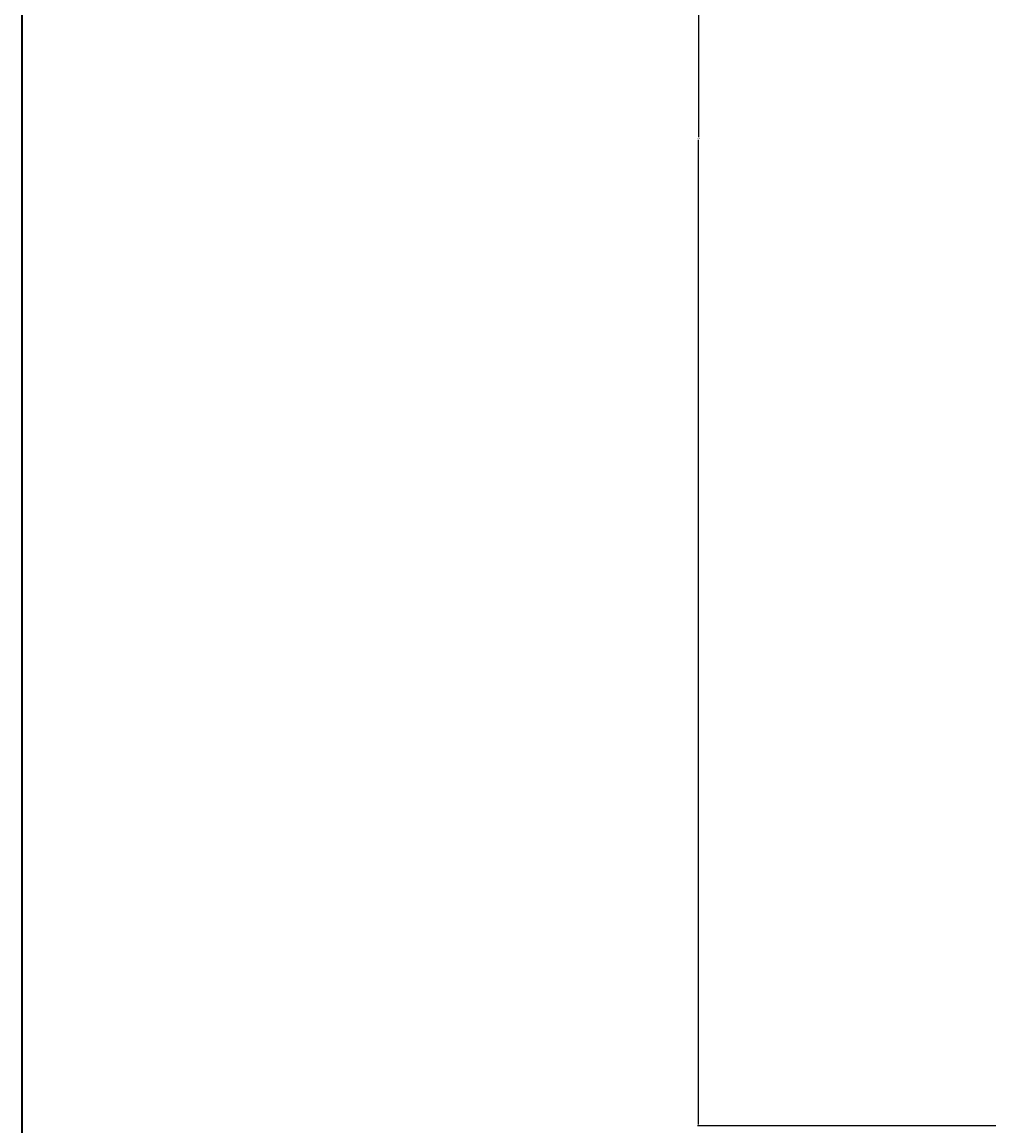
# Model space of a CAD drawing. Units: inches. Extents: x 2120 to 4013, y 1390 to 3019.
# Tile 1 of 59: x 2120 to 2259, y 1582 to 1740. Entities that reach past the tile are written whole.
import ezdxf

# ---------------------------------------------------------------- set-up
doc = ezdxf.new("R2010")
doc.units = ezdxf.units.IN
doc.layers.add('A-ANNO-DIMS', color=2, linetype='Continuous', lineweight=18)
doc.layers.add('A-ANNO-TTLB', color=7, linetype='Continuous', lineweight=35)
doc.styles.get("Standard").update_dxf_attribs({"font": 'arial.ttf'})
doc.dimstyles.get("Standard").update_dxf_attribs({"dimtxt": 0.18, "dimasz": 0.18, "dimexe": 0.18, "dimexo": 0.0625, "dimgap": 0.09, "dimtad": 0, "dimtih": 1, "dimtoh": 1, "dimdec": 4, "dimzin": 0, "dimdsep": 46, "dimtxsty": 'Standard', "dimcen": 0.09, "dimadec": 0, "dimazin": 0, "dimtfac": 1, "dimtdec": 4, "dimtofl": 0, "dimtmove": 0, "dimatfit": 3, "dimfxl": 1, "dimtolj": 1, "dimtzin": 0, "dimarcsym": 0})

# ---------------------------------------------------------------- blocks, each defined once
blk = doc.blocks.new('*D213')
at = {"layer": 'A-ANNO-DIMS', "color": 0, "lineweight": -2, "transparency": 16777216}
for p, q in [((2271.67, 1865.53), (2217.55, 1865.53)), ((2217.73, 1865.35), (2217.73, 1723.71)), ((2217.73, 1581.71), (2217.73, 1723.35)), ((2262.67, 1581.53), (2217.55, 1581.53))]:
    blk.add_line(p, q, dxfattribs=at)
at = {"layer": 'A-ANNO-DIMS', "color": 0, "transparency": 16777216}
for points in [[(2217.7, 1865.35), (2217.76, 1865.35), (2217.73, 1865.53)], [(2217.7, 1581.71), (2217.76, 1581.71), (2217.73, 1581.53)]]:
    blk.add_solid(points, dxfattribs=at)
at = {"layer": 'Defpoints', "color": 0, "transparency": 16777216}
for p in [(2217.73, 1865.53), (2271.73, 1865.53), (2262.73, 1581.53)]:
    blk.add_point(p, dxfattribs=at)
at = {"layer": 'A-ANNO-DIMS', "color": 0, "transparency": 16777216, "insert": (2217.73, 1723.53), "char_height": 0.18, "attachment_point": 5}
blk.add_mtext('\\A1;284', dxfattribs=at)

msp = doc.modelspace()

# ---------------------------------------------------------------- linework, layer by layer
at = {"layer": 'A-ANNO-TTLB'}
msp.add_lwpolyline([(2120.4581, 3019.1237), (4012.9334, 3019.1237), (4012.9334, 1390.2222), (2120.4581, 1390.2222)], close=True, dxfattribs=at)

# ---------------------------------------------------------------- dimensions: what is measured, and where the dimension line sits
at = {"layer": 'A-ANNO-DIMS'}
dim = msp.add_linear_dim(base=(2217.7331, 1865.531), p1=(2262.7331, 1581.531), p2=(2271.7331, 1865.531), angle=90, dimstyle='Standard', override={"dimdec": 0, "dimlfac": 1, "dimrnd": 0, "dimzin": 0, "dimdsep": 46, "dimlunit": 2}, dxfattribs=at)
dim.commit()
dim.dimension.update_dxf_attribs({"geometry": '*D213', "text_midpoint": (2217.7331, 1723.531)})

doc.saveas('drawing.dxf')
